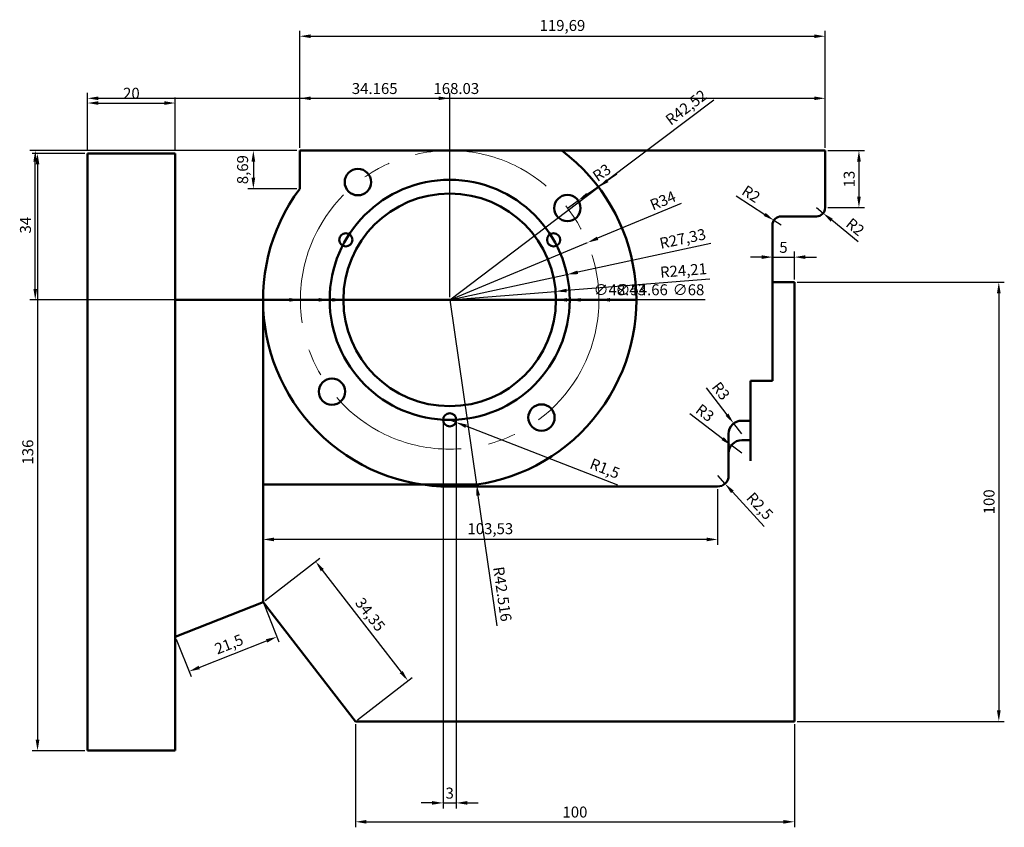
# Model space of a CAD drawing. Units: millimetres. Extents: x 1194 to 1920, y 1729 to 2086.
# Tile 4 of 5: x 1485 to 1709, y 1898 to 2082. Entities that reach past the tile are written whole.
import ezdxf

# ---------------------------------------------------------------- set-up
doc = ezdxf.new("R2010")
doc.units = ezdxf.units.MM
doc.linetypes.add('CENTER', pattern=[50.8, 31.75, -6.35, 6.35, -6.35])
for name, color, linetype, lineweight in [('M-CNTR', 1, 'CENTER', 18), ('M-DIMS', 2, 'Continuous', 25), ('M-OUTL', 7, 'Continuous', 50)]:
    doc.layers.add(name, color=color, linetype=linetype, lineweight=lineweight)
doc.styles.get("Standard").update_dxf_attribs({"font": 'arial.ttf'})
doc.dimstyles.new('ISO-25', dxfattribs={"dimtxt": 2.5, "dimasz": 2.5, "dimexe": 1.25, "dimexo": 0.625, "dimtad": 1, "dimtxsty": 'Standard', "dimcen": 2.5, "dimadec": 0, "dimazin": 0, "dimtfac": 1, "dimtmove": 0, "dimatfit": 3, "dimfxl": 1, "dimarcsym": 0})

# ---------------------------------------------------------------- blocks, each defined once
blk = doc.blocks.new('*U5')
blk.add_circle((0, 0), 1.5)
blk = doc.blocks.new('*U6')
at = {"layer": 'M-OUTL', "color": 0, "linetype": 'ByBlock', "lineweight": -2, "transparency": 16777216}
for p, rotation in [((1558.99, 2031.94), 240), ((1606.33, 2031.94), 119.9999999999999)]:
    blk.add_blockref('*U5', p, dxfattribs=dict(at, rotation=rotation))
blk.add_blockref('*U5', (1582.66, 1990.95), dxfattribs=at)
blk = doc.blocks.new('*U7')
blk.add_circle((0, 0), 3)
blk = doc.blocks.new('*U8')
at = {"layer": 'M-OUTL', "color": 0, "linetype": 'ByBlock', "lineweight": -2, "transparency": 16777216}
for p, rotation in [((1561.75, 2045.09), 90), ((1555.85, 1997.37), 180), ((1603.57, 1991.47), 270)]:
    blk.add_blockref('*U7', p, dxfattribs=dict(at, rotation=rotation))
blk.add_blockref('*U7', (1609.47, 2039.19), dxfattribs=at)
blk = doc.blocks.new('*D40')
at = {"layer": 'Defpoints', "color": 0, "transparency": 16777216}
for p in [(1500.16, 2051.61), (1488.78, 1915.61), (1500.16, 1915.61)]:
    blk.add_point(p, dxfattribs=at)
at = {"layer": 'M-DIMS', "color": 0, "lineweight": -2, "transparency": 16777216}
for p, q in [((1499.54, 2051.61), (1487.53, 2051.61)), ((1488.78, 2049.11), (1488.78, 1918.11)), ((1499.54, 1915.61), (1487.53, 1915.61))]:
    blk.add_line(p, q, dxfattribs=at)
at = {"layer": 'M-DIMS', "color": 0, "transparency": 16777216}
for points in [[(1488.36, 2049.11), (1489.2, 2049.11), (1488.78, 2051.61)], [(1488.36, 1918.11), (1489.2, 1918.11), (1488.78, 1915.61)]]:
    blk.add_solid(points, dxfattribs=at)
at = {"layer": 'M-DIMS', "color": 0, "transparency": 16777216, "insert": (1486.88, 1983.61), "char_height": 2.5, "attachment_point": 5, "rotation": 90}
blk.add_mtext('136', dxfattribs=at)
blk = doc.blocks.new('*D41')
at = {"layer": 'Defpoints', "color": 0, "transparency": 16777216}
for p in [(1520.16, 2063.1), (1500.16, 2051.61), (1520.16, 2051.61)]:
    blk.add_point(p, dxfattribs=at)
at = {"layer": 'M-DIMS', "color": 0, "lineweight": -2, "transparency": 16777216}
for p, q in [((1500.16, 2052.24), (1500.16, 2064.35)), ((1520.16, 2052.24), (1520.16, 2064.35)), ((1502.66, 2063.1), (1517.66, 2063.1))]:
    blk.add_line(p, q, dxfattribs=at)
at = {"layer": 'M-DIMS', "color": 0, "transparency": 16777216}
for points in [[(1502.66, 2063.51), (1502.66, 2062.68), (1500.16, 2063.1)], [(1517.66, 2063.51), (1517.66, 2062.68), (1520.16, 2063.1)]]:
    blk.add_solid(points, dxfattribs=at)
at = {"layer": 'M-DIMS', "color": 0, "transparency": 16777216, "insert": (1510.16, 2065), "char_height": 2.5, "attachment_point": 5}
blk.add_mtext('20', dxfattribs=at)
blk = doc.blocks.new('*D42')
at = {"layer": 'Defpoints', "color": 0, "transparency": 16777216}
for p in [(1540.16, 1949.44), (1520.16, 1941.56), (1543.28, 1941.52)]:
    blk.add_point(p, dxfattribs=at)
at = {"layer": 'M-DIMS', "color": 0, "lineweight": -2, "transparency": 16777216}
for p, q in [((1540.39, 1948.86), (1543.74, 1940.36)), ((1520.39, 1940.97), (1523.74, 1932.48)), ((1525.61, 1934.56), (1540.96, 1940.61))]:
    blk.add_line(p, q, dxfattribs=at)
at = {"layer": 'M-DIMS', "color": 0, "transparency": 16777216}
for points in [[(1540.8, 1941), (1541.11, 1940.22), (1543.28, 1941.52)], [(1525.46, 1934.94), (1525.76, 1934.17), (1523.28, 1933.64)]]:
    blk.add_solid(points, dxfattribs=at)
at = {"layer": 'M-DIMS', "color": 0, "transparency": 16777216, "insert": (1532.5, 1939.56), "char_height": 2.5, "attachment_point": 5, "rotation": 21.5204}
blk.add_mtext('21,5', dxfattribs=at)
blk = doc.blocks.new('*D43')
at = {"layer": 'Defpoints', "color": 0, "transparency": 16777216}
for p in [(1540.16, 1949.44), (1573.15, 1931.54), (1561.19, 1922.28)]:
    blk.add_point(p, dxfattribs=at)
at = {"layer": 'M-DIMS', "color": 0, "lineweight": -2, "transparency": 16777216}
for p, q in [((1540.66, 1949.82), (1553.11, 1959.46)), ((1553.65, 1956.72), (1571.62, 1933.51)), ((1561.68, 1922.66), (1574.14, 1932.3))]:
    blk.add_line(p, q, dxfattribs=at)
at = {"layer": 'M-DIMS', "color": 0, "transparency": 16777216}
for points in [[(1553.98, 1956.98), (1553.32, 1956.47), (1552.12, 1958.7)], [(1571.95, 1933.77), (1571.29, 1933.26), (1573.15, 1931.54)]]:
    blk.add_solid(points, dxfattribs=at)
at = {"layer": 'M-DIMS', "color": 0, "transparency": 16777216, "insert": (1564.32, 1946.42), "char_height": 2.5, "attachment_point": 5, "rotation": 307.7411}
blk.add_mtext('34,35', dxfattribs=at)
blk = doc.blocks.new('*D44')
at = {"layer": 'Defpoints', "color": 0, "transparency": 16777216}
for p in [(1561.19, 1922.28), (1661.19, 1922.28), (1661.19, 1899.41)]:
    blk.add_point(p, dxfattribs=at)
at = {"layer": 'M-DIMS', "color": 0, "lineweight": -2, "transparency": 16777216}
for p, q in [((1561.19, 1921.65), (1561.19, 1898.16)), ((1661.19, 1921.65), (1661.19, 1898.16)), ((1563.69, 1899.41), (1658.69, 1899.41))]:
    blk.add_line(p, q, dxfattribs=at)
at = {"layer": 'M-DIMS', "color": 0, "transparency": 16777216}
for points in [[(1563.69, 1899.82), (1563.69, 1898.99), (1561.19, 1899.41)], [(1658.69, 1899.82), (1658.69, 1898.99), (1661.19, 1899.41)]]:
    blk.add_solid(points, dxfattribs=at)
at = {"layer": 'M-DIMS', "color": 0, "transparency": 16777216, "insert": (1611.19, 1901.31), "char_height": 2.5, "attachment_point": 5}
blk.add_mtext('100', dxfattribs=at)
blk = doc.blocks.new('*D45')
at = {"layer": 'Defpoints', "color": 0, "transparency": 16777216}
for p in [(1668.19, 2078.31), (1548.5, 2052.28), (1668.19, 2052.28)]:
    blk.add_point(p, dxfattribs=at)
at = {"layer": 'M-DIMS', "color": 0, "lineweight": -2, "transparency": 16777216}
for p, q in [((1548.5, 2052.9), (1548.5, 2079.56)), ((1668.19, 2052.9), (1668.19, 2079.56)), ((1551, 2078.31), (1665.69, 2078.31))]:
    blk.add_line(p, q, dxfattribs=at)
at = {"layer": 'M-DIMS', "color": 0, "transparency": 16777216}
for points in [[(1551, 2078.73), (1551, 2077.89), (1548.5, 2078.31)], [(1665.69, 2078.73), (1665.69, 2077.89), (1668.19, 2078.31)]]:
    blk.add_solid(points, dxfattribs=at)
at = {"layer": 'M-DIMS', "color": 0, "transparency": 16777216, "insert": (1608.34, 2080.44), "char_height": 2.5, "attachment_point": 5}
blk.add_mtext('119,69', dxfattribs=at)
blk = doc.blocks.new('*D46')
at = {"layer": 'Defpoints', "color": 0, "transparency": 16777216}
for p in [(1668.19, 2052.28), (1668.19, 2039.28), (1675.88, 2039.28)]:
    blk.add_point(p, dxfattribs=at)
at = {"layer": 'M-DIMS', "color": 0, "lineweight": -2, "transparency": 16777216}
for p, q in [((1668.81, 2052.28), (1677.13, 2052.28)), ((1675.88, 2049.78), (1675.88, 2041.78)), ((1668.81, 2039.28), (1677.13, 2039.28))]:
    blk.add_line(p, q, dxfattribs=at)
at = {"layer": 'M-DIMS', "color": 0, "transparency": 16777216}
for points in [[(1675.46, 2049.78), (1676.3, 2049.78), (1675.88, 2052.28)], [(1675.46, 2041.78), (1676.3, 2041.78), (1675.88, 2039.28)]]:
    blk.add_solid(points, dxfattribs=at)
at = {"layer": 'M-DIMS', "color": 0, "transparency": 16777216, "insert": (1673.98, 2045.78), "char_height": 2.5, "attachment_point": 5, "rotation": 90}
blk.add_mtext('13', dxfattribs=at)
blk = doc.blocks.new('*D47')
at = {"layer": 'Defpoints', "color": 0, "transparency": 16777216}
for p in [(1666.19, 2039.28), (1667.73, 2038.01)]:
    blk.add_point(p, dxfattribs=at)
at = {"layer": 'M-DIMS', "color": 0, "lineweight": -2, "transparency": 16777216}
for p, q in [((1666.19, 2039.28), (1667.73, 2038.01)), ((1675.67, 2031.51), (1669.67, 2036.43))]:
    blk.add_line(p, q, dxfattribs=at)
at = {"layer": 'M-DIMS', "color": 0, "transparency": 16777216}
blk.add_solid([(1669.93, 2036.75), (1669.4, 2036.1), (1667.73, 2038.01)], dxfattribs=at)
at = {"layer": 'M-DIMS', "color": 0, "transparency": 16777216, "insert": (1674.83, 2034.63), "char_height": 2.5, "attachment_point": 5, "rotation": 320.6916}
blk.add_mtext('R2', dxfattribs=at)
blk = doc.blocks.new('*D48')
at = {"layer": 'Defpoints', "color": 0, "transparency": 16777216}
for p in [(1656.51, 2036.37), (1658.19, 2035.28)]:
    blk.add_point(p, dxfattribs=at)
at = {"layer": 'M-DIMS', "color": 0, "lineweight": -2, "transparency": 16777216}
for p, q in [((1647.92, 2041.98), (1654.42, 2037.74)), ((1658.19, 2035.28), (1656.51, 2036.37))]:
    blk.add_line(p, q, dxfattribs=at)
at = {"layer": 'M-DIMS', "color": 0, "transparency": 16777216}
blk.add_solid([(1654.65, 2038.09), (1654.19, 2037.39), (1656.51, 2036.37)], dxfattribs=at)
at = {"layer": 'M-DIMS', "color": 0, "transparency": 16777216, "insert": (1651.15, 2042.12), "char_height": 2.5, "attachment_point": 5, "rotation": 326.8616}
blk.add_mtext('R2', dxfattribs=at)
blk = doc.blocks.new('*D49')
at = {"layer": 'Defpoints', "color": 0, "transparency": 16777216}
for p in [(1661.19, 2022.28), (1661.19, 1922.28), (1707.74, 1922.28)]:
    blk.add_point(p, dxfattribs=at)
at = {"layer": 'M-DIMS', "color": 0, "lineweight": -2, "transparency": 16777216}
for p, q in [((1661.81, 2022.28), (1708.99, 2022.28)), ((1707.74, 2019.78), (1707.74, 1924.78)), ((1661.81, 1922.28), (1708.99, 1922.28))]:
    blk.add_line(p, q, dxfattribs=at)
at = {"layer": 'M-DIMS', "color": 0, "transparency": 16777216}
for points in [[(1707.32, 2019.78), (1708.16, 2019.78), (1707.74, 2022.28)], [(1707.32, 1924.78), (1708.16, 1924.78), (1707.74, 1922.28)]]:
    blk.add_solid(points, dxfattribs=at)
at = {"layer": 'M-DIMS', "color": 0, "transparency": 16777216, "insert": (1705.84, 1972.28), "char_height": 2.5, "attachment_point": 5, "rotation": 90}
blk.add_mtext('100', dxfattribs=at)
blk = doc.blocks.new('*D50')
at = {"layer": 'Defpoints', "color": 0, "transparency": 16777216}
for p in [(1661.19, 2028.01), (1656.19, 2022.28), (1661.19, 2022.28)]:
    blk.add_point(p, dxfattribs=at)
at = {"layer": 'M-DIMS', "color": 0, "lineweight": -2, "transparency": 16777216}
for p, q in [((1653.69, 2028.01), (1651.19, 2028.01)), ((1656.19, 2022.9), (1656.19, 2029.26)), ((1656.19, 2028.01), (1661.19, 2028.01)), ((1661.19, 2022.9), (1661.19, 2029.26)), ((1663.69, 2028.01), (1666.19, 2028.01))]:
    blk.add_line(p, q, dxfattribs=at)
at = {"layer": 'M-DIMS', "color": 0, "transparency": 16777216}
for points in [[(1653.69, 2028.43), (1653.69, 2027.59), (1656.19, 2028.01)], [(1663.69, 2028.43), (1663.69, 2027.59), (1661.19, 2028.01)]]:
    blk.add_solid(points, dxfattribs=at)
at = {"layer": 'M-DIMS', "color": 0, "transparency": 16777216, "insert": (1658.69, 2029.91), "char_height": 2.5, "attachment_point": 5}
blk.add_mtext('5', dxfattribs=at)
blk = doc.blocks.new('*D51')
at = {"layer": 'Defpoints', "color": 0, "transparency": 16777216}
for p in [(1540.16, 1976.21), (1643.69, 1975.76), (1540.16, 1963.71)]:
    blk.add_point(p, dxfattribs=at)
at = {"layer": 'M-DIMS', "color": 0, "lineweight": -2, "transparency": 16777216}
for p, q in [((1540.16, 1975.58), (1540.16, 1962.46)), ((1643.69, 1975.14), (1643.69, 1962.46)), ((1641.19, 1963.71), (1542.66, 1963.71))]:
    blk.add_line(p, q, dxfattribs=at)
at = {"layer": 'M-DIMS', "color": 0, "transparency": 16777216}
for points in [[(1542.66, 1964.13), (1542.66, 1963.29), (1540.16, 1963.71)], [(1641.19, 1964.13), (1641.19, 1963.29), (1643.69, 1963.71)]]:
    blk.add_solid(points, dxfattribs=at)
at = {"layer": 'M-DIMS', "color": 0, "transparency": 16777216, "insert": (1591.92, 1965.84), "char_height": 2.5, "attachment_point": 5}
blk.add_mtext('103,53', dxfattribs=at)
blk = doc.blocks.new('*D52')
at = {"layer": 'Defpoints', "color": 0, "transparency": 16777216}
for p in [(1647.35, 1990.14), (1649.19, 1987.76)]:
    blk.add_point(p, dxfattribs=at)
at = {"layer": 'M-DIMS', "color": 0, "lineweight": -2, "transparency": 16777216}
for p, q in [((1641.06, 1998.27), (1645.82, 1992.11)), ((1649.19, 1987.76), (1647.35, 1990.14))]:
    blk.add_line(p, q, dxfattribs=at)
at = {"layer": 'M-DIMS', "color": 0, "transparency": 16777216}
blk.add_solid([(1646.15, 1992.37), (1645.49, 1991.86), (1647.35, 1990.14)], dxfattribs=at)
at = {"layer": 'M-DIMS', "color": 0, "transparency": 16777216, "insert": (1644.18, 1997.34), "char_height": 2.5, "attachment_point": 5, "rotation": 307.7239}
blk.add_mtext('R3', dxfattribs=at)
blk = doc.blocks.new('*D53')
at = {"layer": 'Defpoints', "color": 0, "transparency": 16777216}
for p in [(1646.81, 1985.15), (1649.19, 1983.33)]:
    blk.add_point(p, dxfattribs=at)
at = {"layer": 'M-DIMS', "color": 0, "lineweight": -2, "transparency": 16777216}
for p, q in [((1637.36, 1992.39), (1644.82, 1986.67)), ((1649.19, 1983.33), (1646.81, 1985.15))]:
    blk.add_line(p, q, dxfattribs=at)
at = {"layer": 'M-DIMS', "color": 0, "transparency": 16777216}
blk.add_solid([(1645.07, 1987), (1644.57, 1986.34), (1646.81, 1985.15)], dxfattribs=at)
at = {"layer": 'M-DIMS', "color": 0, "transparency": 16777216, "insert": (1640.61, 1992.29), "char_height": 2.5, "attachment_point": 5, "rotation": 322.5412}
blk.add_mtext('R3', dxfattribs=at)
blk = doc.blocks.new('*D54')
at = {"layer": 'Defpoints', "color": 0, "transparency": 16777216}
for p in [(1643.69, 1978.26), (1645.37, 1976.41)]:
    blk.add_point(p, dxfattribs=at)
at = {"layer": 'M-DIMS', "color": 0, "lineweight": -2, "transparency": 16777216}
for p, q in [((1643.69, 1978.26), (1645.37, 1976.41)), ((1654.26, 1966.64), (1647.05, 1974.56))]:
    blk.add_line(p, q, dxfattribs=at)
at = {"layer": 'M-DIMS', "color": 0, "transparency": 16777216}
blk.add_solid([(1647.36, 1974.84), (1646.74, 1974.28), (1645.37, 1976.41)], dxfattribs=at)
at = {"layer": 'M-DIMS', "color": 0, "transparency": 16777216, "insert": (1653.07, 1971.11), "char_height": 2.5, "attachment_point": 5, "rotation": 312.2746}
blk.add_mtext('R2,5', dxfattribs=at)
blk = doc.blocks.new('*D55')
at = {"layer": 'Defpoints', "color": 0, "transparency": 16777216}
for p in [(1616.57, 2043.93), (1582.66, 2018.28)]:
    blk.add_point(p, dxfattribs=at)
at = {"layer": 'M-DIMS', "color": 0, "lineweight": -2, "transparency": 16777216}
for p, q in [((1642.81, 2063.78), (1618.56, 2045.44)), ((1582.66, 2018.28), (1616.57, 2043.93))]:
    blk.add_line(p, q, dxfattribs=at)
at = {"layer": 'M-DIMS', "color": 0, "transparency": 16777216}
blk.add_solid([(1618.31, 2045.77), (1618.81, 2045.1), (1616.57, 2043.93)], dxfattribs=at)
at = {"layer": 'M-DIMS', "color": 0, "transparency": 16777216, "insert": (1636.72, 2061.84), "char_height": 2.5, "attachment_point": 5, "rotation": 37.1061}
blk.add_mtext('R42,52', dxfattribs=at)
blk = doc.blocks.new('*D56')
at = {"layer": 'Defpoints', "color": 0, "transparency": 16777216}
for p in [(1614.06, 2031.33), (1582.66, 2018.28)]:
    blk.add_point(p, dxfattribs=at)
at = {"layer": 'M-DIMS', "color": 0, "lineweight": -2, "transparency": 16777216}
for p, q in [((1635.4, 2040.21), (1616.36, 2032.29)), ((1582.66, 2018.28), (1614.06, 2031.33))]:
    blk.add_line(p, q, dxfattribs=at)
at = {"layer": 'M-DIMS', "color": 0, "transparency": 16777216}
blk.add_solid([(1616.2, 2032.68), (1616.52, 2031.91), (1614.06, 2031.33)], dxfattribs=at)
at = {"layer": 'M-DIMS', "color": 0, "transparency": 16777216, "insert": (1631.34, 2040.58), "char_height": 2.5, "attachment_point": 5, "rotation": 22.5772}
blk.add_mtext('R34', dxfattribs=at)
blk = doc.blocks.new('*D57')
at = {"layer": 'Defpoints', "color": 0, "transparency": 16777216}
for p in [(1609.38, 2024.03), (1582.66, 2018.28)]:
    blk.add_point(p, dxfattribs=at)
at = {"layer": 'M-DIMS', "color": 0, "lineweight": -2, "transparency": 16777216}
for p, q in [((1642.15, 2031.08), (1611.82, 2024.55)), ((1582.66, 2018.28), (1609.38, 2024.03))]:
    blk.add_line(p, q, dxfattribs=at)
at = {"layer": 'M-DIMS', "color": 0, "transparency": 16777216}
blk.add_solid([(1611.74, 2024.96), (1611.91, 2024.14), (1609.38, 2024.03)], dxfattribs=at)
at = {"layer": 'M-DIMS', "color": 0, "transparency": 16777216, "insert": (1635.8, 2031.89), "char_height": 2.5, "attachment_point": 5, "rotation": 12.1415}
blk.add_mtext('R27,33', dxfattribs=at)
blk = doc.blocks.new('*D58')
at = {"layer": 'Defpoints', "color": 0, "transparency": 16777216}
for p in [(1606.8, 2020.2), (1582.66, 2018.28)]:
    blk.add_point(p, dxfattribs=at)
at = {"layer": 'M-DIMS', "color": 0, "lineweight": -2, "transparency": 16777216}
for p, q in [((1641.89, 2023), (1609.29, 2020.4)), ((1582.66, 2018.28), (1606.8, 2020.2))]:
    blk.add_line(p, q, dxfattribs=at)
at = {"layer": 'M-DIMS', "color": 0, "transparency": 16777216}
blk.add_solid([(1609.26, 2020.82), (1609.32, 2019.99), (1606.8, 2020.2)], dxfattribs=at)
at = {"layer": 'M-DIMS', "color": 0, "transparency": 16777216, "insert": (1635.94, 2024.66), "char_height": 2.5, "attachment_point": 5, "rotation": 4.5586}
blk.add_mtext('R24,21', dxfattribs=at)
blk = doc.blocks.new('*D59')
at = {"layer": 'Defpoints', "color": 0, "transparency": 16777216}
for p in [(1611.94, 2040.89), (1609.47, 2039.19)]:
    blk.add_point(p, dxfattribs=at)
at = {"layer": 'M-DIMS', "color": 0, "lineweight": -2, "transparency": 16777216}
for p, q in [((1620.74, 2046.93), (1614, 2042.3)), ((1609.47, 2039.19), (1611.94, 2040.89))]:
    blk.add_line(p, q, dxfattribs=at)
at = {"layer": 'M-DIMS', "color": 0, "transparency": 16777216}
blk.add_solid([(1613.77, 2042.65), (1614.24, 2041.96), (1611.94, 2040.89)], dxfattribs=at)
at = {"layer": 'M-DIMS', "color": 0, "transparency": 16777216, "insert": (1617.48, 2047), "char_height": 2.5, "attachment_point": 5, "rotation": 34.5057}
blk.add_mtext('R3', dxfattribs=at)
blk = doc.blocks.new('*D60')
at = {"layer": 'Defpoints', "color": 0, "transparency": 16777216}
for p in [(1582.66, 1990.95), (1584.06, 1990.4)]:
    blk.add_point(p, dxfattribs=at)
at = {"layer": 'M-DIMS', "color": 0, "lineweight": -2, "transparency": 16777216}
for p, q in [((1582.66, 1990.95), (1584.06, 1990.4)), ((1620.95, 1976.11), (1586.39, 1989.5))]:
    blk.add_line(p, q, dxfattribs=at)
at = {"layer": 'M-DIMS', "color": 0, "transparency": 16777216}
blk.add_solid([(1586.54, 1989.89), (1586.24, 1989.11), (1584.06, 1990.4)], dxfattribs=at)
at = {"layer": 'M-DIMS', "color": 0, "transparency": 16777216, "insert": (1617.89, 1979.58), "char_height": 2.5, "attachment_point": 5, "rotation": 338.8182}
blk.add_mtext('R1,5', dxfattribs=at)
blk = doc.blocks.new('*D61')
at = {"layer": 'Defpoints', "color": 0, "transparency": 16777216}
for p in [(1548.5, 2052.28), (1537.94, 2043.58), (1548.5, 2043.58)]:
    blk.add_point(p, dxfattribs=at)
at = {"layer": 'M-DIMS', "color": 0, "lineweight": -2, "transparency": 16777216}
for p, q in [((1547.87, 2052.28), (1536.69, 2052.28)), ((1537.94, 2049.78), (1537.94, 2046.08)), ((1547.87, 2043.58), (1536.69, 2043.58))]:
    blk.add_line(p, q, dxfattribs=at)
at = {"layer": 'M-DIMS', "color": 0, "transparency": 16777216}
for points in [[(1537.53, 2049.78), (1538.36, 2049.78), (1537.94, 2052.28)], [(1537.53, 2046.08), (1538.36, 2046.08), (1537.94, 2043.58)]]:
    blk.add_solid(points, dxfattribs=at)
at = {"layer": 'M-DIMS', "color": 0, "transparency": 16777216, "insert": (1535.82, 2047.93), "char_height": 2.5, "attachment_point": 5, "rotation": 90}
blk.add_mtext('8,69', dxfattribs=at)
blk = doc.blocks.new('*D137')
at = {"layer": 'Defpoints', "color": 0, "transparency": 16777216}
for p in [(1581.16, 1990.95), (1584.16, 1990.95), (1584.16, 1903.71)]:
    blk.add_point(p, dxfattribs=at)
at = {"layer": 'M-DIMS', "color": 0, "lineweight": -2, "transparency": 16777216}
for p, q in [((1581.16, 1990.32), (1581.16, 1902.46)), ((1584.16, 1990.32), (1584.16, 1902.46)), ((1578.66, 1903.71), (1576.16, 1903.71)), ((1581.16, 1903.71), (1584.16, 1903.71)), ((1586.66, 1903.71), (1589.16, 1903.71))]:
    blk.add_line(p, q, dxfattribs=at)
at = {"layer": 'M-DIMS', "color": 0, "transparency": 16777216}
for points in [[(1578.66, 1904.13), (1578.66, 1903.3), (1581.16, 1903.71)], [(1586.66, 1904.13), (1586.66, 1903.3), (1584.16, 1903.71)]]:
    blk.add_solid(points, dxfattribs=at)
at = {"layer": 'M-DIMS', "color": 0, "transparency": 16777216, "insert": (1582.66, 1905.62), "char_height": 2.5, "attachment_point": 5}
blk.add_mtext('3', dxfattribs=at)
blk = doc.blocks.new('*D139')
at = {"layer": 'Defpoints', "color": 0, "transparency": 16777216}
for p in [(1668.19, 2064.18), (1668.19, 2052.28), (1500.16, 2051.61)]:
    blk.add_point(p, dxfattribs=at)
at = {"layer": 'M-DIMS', "color": 0, "lineweight": -2, "transparency": 16777216}
for p, q in [((1500.16, 2052.24), (1500.16, 2065.43)), ((1502.66, 2064.18), (1665.69, 2064.18)), ((1668.19, 2052.9), (1668.19, 2065.43))]:
    blk.add_line(p, q, dxfattribs=at)
at = {"layer": 'M-DIMS', "color": 0, "transparency": 16777216}
for points in [[(1502.66, 2064.59), (1502.66, 2063.76), (1500.16, 2064.18)], [(1665.69, 2064.59), (1665.69, 2063.76), (1668.19, 2064.18)]]:
    blk.add_solid(points, dxfattribs=at)
at = {"layer": 'M-DIMS', "color": 0, "transparency": 16777216, "insert": (1584.17, 2066.08), "char_height": 2.5, "attachment_point": 5}
blk.add_mtext('168.03', dxfattribs=at)
blk = doc.blocks.new('*D140')
at = {"layer": 'Defpoints', "color": 0, "transparency": 16777216}
for p in [(1582.66, 2064.18), (1548.5, 2052.28), (1582.66, 2018.28)]:
    blk.add_point(p, dxfattribs=at)
at = {"layer": 'M-DIMS', "color": 0, "lineweight": -2, "transparency": 16777216}
for p, q in [((1548.5, 2052.9), (1548.5, 2065.43)), ((1551, 2064.18), (1580.16, 2064.18)), ((1582.66, 2018.9), (1582.66, 2065.43))]:
    blk.add_line(p, q, dxfattribs=at)
at = {"layer": 'M-DIMS', "color": 0, "transparency": 16777216}
for points in [[(1551, 2064.59), (1551, 2063.76), (1548.5, 2064.18)], [(1580.16, 2064.59), (1580.16, 2063.76), (1582.66, 2064.18)]]:
    blk.add_solid(points, dxfattribs=at)
at = {"layer": 'M-DIMS', "color": 0, "transparency": 16777216, "insert": (1565.58, 2066.08), "char_height": 2.5, "attachment_point": 5}
blk.add_mtext('34.165', dxfattribs=at)
blk = doc.blocks.new('*D141')
at = {"layer": 'Defpoints', "color": 0, "transparency": 16777216}
for p in [(1488.26, 2052.28), (1548.5, 2052.28), (1582.66, 2018.28)]:
    blk.add_point(p, dxfattribs=at)
at = {"layer": 'M-DIMS', "color": 0, "lineweight": -2, "transparency": 16777216}
for p, q in [((1547.87, 2052.28), (1487.01, 2052.28)), ((1488.26, 2020.78), (1488.26, 2049.78)), ((1582.04, 2018.28), (1487.01, 2018.28))]:
    blk.add_line(p, q, dxfattribs=at)
at = {"layer": 'M-DIMS', "color": 0, "transparency": 16777216}
for points in [[(1487.84, 2049.78), (1488.68, 2049.78), (1488.26, 2052.28)], [(1487.84, 2020.78), (1488.68, 2020.78), (1488.26, 2018.28)]]:
    blk.add_solid(points, dxfattribs=at)
at = {"layer": 'M-DIMS', "color": 0, "transparency": 16777216, "insert": (1486.36, 2035.28), "char_height": 2.5, "attachment_point": 5, "rotation": 90}
blk.add_mtext('34', dxfattribs=at)
blk = doc.blocks.new('*D145')
at = {"layer": 'Defpoints', "color": 0, "transparency": 16777216}
for p in [(1582.66, 2018.28), (1588.79, 1976.21)]:
    blk.add_point(p, dxfattribs=at)
at = {"layer": 'M-DIMS', "color": 0, "lineweight": -2, "transparency": 16777216}
for p, q in [((1582.66, 2018.28), (1588.79, 1976.21)), ((1593.48, 1944.03), (1589.15, 1973.73))]:
    blk.add_line(p, q, dxfattribs=at)
at = {"layer": 'M-DIMS', "color": 0, "transparency": 16777216}
blk.add_solid([(1589.56, 1973.79), (1588.74, 1973.67), (1588.79, 1976.21)], dxfattribs=at)
at = {"layer": 'M-DIMS', "color": 0, "transparency": 16777216, "insert": (1594.35, 1951.24), "char_height": 2.5, "attachment_point": 5, "rotation": 278.2873}
blk.add_mtext('R42.516', dxfattribs=at)
blk = doc.blocks.new('*D146')
at = {"layer": 'Defpoints', "color": 0, "transparency": 16777216}
for p in [(1548.66, 2018.28), (1616.66, 2018.28)]:
    blk.add_point(p, dxfattribs=at)
at = {"layer": 'M-DIMS', "color": 0, "lineweight": -2, "transparency": 16777216}
for p, q in [((1546.16, 2018.28), (1543.66, 2018.28)), ((1548.66, 2018.28), (1616.66, 2018.28)), ((1640.84, 2018.28), (1619.16, 2018.28))]:
    blk.add_line(p, q, dxfattribs=at)
at = {"layer": 'M-DIMS', "color": 0, "transparency": 16777216}
for points in [[(1546.16, 2018.69), (1546.16, 2017.86), (1548.66, 2018.28)], [(1619.16, 2018.69), (1619.16, 2017.86), (1616.66, 2018.28)]]:
    blk.add_solid(points, dxfattribs=at)
at = {"layer": 'M-DIMS', "color": 0, "transparency": 16777216, "insert": (1637.06, 2020.25), "char_height": 2.5, "attachment_point": 5, "rotation": 0.0001}
blk.add_mtext('∅68', dxfattribs=at)
blk = doc.blocks.new('*D147')
at = {"layer": 'Defpoints', "color": 0, "transparency": 16777216}
for p in [(1555.33, 2018.28), (1609.99, 2018.28)]:
    blk.add_point(p, dxfattribs=at)
at = {"layer": 'M-DIMS', "color": 0, "lineweight": -2, "transparency": 16777216}
for p, q in [((1552.83, 2018.28), (1550.33, 2018.28)), ((1555.33, 2018.28), (1609.99, 2018.28)), ((1632.59, 2018.28), (1612.49, 2018.28))]:
    blk.add_line(p, q, dxfattribs=at)
at = {"layer": 'M-DIMS', "color": 0, "transparency": 16777216}
for points in [[(1552.83, 2018.69), (1552.83, 2017.86), (1555.33, 2018.28)], [(1612.49, 2018.69), (1612.49, 2017.86), (1609.99, 2018.28)]]:
    blk.add_solid(points, dxfattribs=at)
at = {"layer": 'M-DIMS', "color": 0, "transparency": 16777216, "insert": (1626.39, 2020.25), "char_height": 2.5, "attachment_point": 5, "rotation": 0.0002}
blk.add_mtext('∅54.66', dxfattribs=at)
blk = doc.blocks.new('*D148')
at = {"layer": 'Defpoints', "color": 0, "transparency": 16777216}
for p in [(1558.45, 2018.28), (1606.88, 2018.28)]:
    blk.add_point(p, dxfattribs=at)
at = {"layer": 'M-DIMS', "color": 0, "lineweight": -2, "transparency": 16777216}
for p, q in [((1555.95, 2018.28), (1553.45, 2018.28)), ((1558.45, 2018.28), (1606.88, 2018.28)), ((1627.61, 2018.28), (1609.38, 2018.28))]:
    blk.add_line(p, q, dxfattribs=at)
at = {"layer": 'M-DIMS', "color": 0, "transparency": 16777216}
for points in [[(1555.95, 2018.69), (1555.95, 2017.86), (1558.45, 2018.28)], [(1609.38, 2018.69), (1609.38, 2017.86), (1606.88, 2018.28)]]:
    blk.add_solid(points, dxfattribs=at)
at = {"layer": 'M-DIMS', "color": 0, "transparency": 16777216, "insert": (1621.4, 2020.25), "char_height": 2.5, "attachment_point": 5, "rotation": 0.0002}
blk.add_mtext('∅48.43', dxfattribs=at)

msp = doc.modelspace()

# ---------------------------------------------------------------- linework, layer by layer
at = {"layer": 'M-CNTR'}
msp.add_circle((1582.6609, 2018.2779), 34, dxfattribs=at)
at = {"layer": 'M-OUTL'}
for p, q in [((1548.4964, 2043.5834), (1548.4964, 2052.2779)), ((1582.6609, 2052.2779), (1548.4964, 2052.2779)), ((1582.6609, 2052.2779), (1608.187, 2052.2779)), ((1608.187, 2052.2779), (1668.187, 2052.2779)), ((1668.187, 2052.2779), (1668.187, 2039.2779)), ((1500.1609, 2051.6148), (1500.1609, 1915.6148)), ((1520.1609, 2051.6148), (1500.1609, 2051.6148)), ((1520.1609, 1915.6148), (1520.1609, 2051.6148)), ((1656.187, 2037.2779), (1656.187, 2037.2779)), ((1666.187, 2037.2779), (1658.187, 2037.2779)), ((1656.187, 2035.2779), (1656.187, 1999.8538)), ((1656.187, 2035.2779), (1656.187, 2022.2779)), ((1656.187, 2022.2779), (1661.187, 2022.2779)), ((1661.187, 2022.2779), (1661.187, 1922.2779)), ((1520.1609, 2018.2779), (1625.1765, 2018.2779)), ((1520.1609, 2018.2779), (1540.1609, 2018.2779)), ((1540.1609, 2018.2779), (1540.1609, 1949.4422)), ((1656.187, 1999.8538), (1651.187, 1999.8538)), ((1651.187, 1999.8538), (1651.187, 1981.5982)), ((1649.187, 1990.7623), (1651.187, 1990.7623)), ((1646.187, 1983.3258), (1646.187, 1987.7623)), ((1649.187, 1986.3258), (1651.187, 1986.3258)), ((1646.187, 1978.2623), (1646.187, 1983.3258)), ((1588.7891, 1976.2063), (1540.1609, 1976.2063)), ((1582.6609, 1975.7623), (1643.687, 1975.7623)), ((1540.1609, 1949.4422), (1520.1609, 1941.5557)), ((1561.187, 1922.2779), (1540.1609, 1949.4422)), ((1661.187, 1922.2779), (1561.187, 1922.2779)), ((1500.1609, 1915.6148), (1520.1609, 1915.6148))]:
    msp.add_line(p, q, dxfattribs=at)
for radius in [27.3311, 24.2146]:
    msp.add_circle((1582.6609, 2018.2779), radius, dxfattribs=at)
for centre, radius, start, end in [((1582.6609, 2018.2779), 42.5156, 143.472882, 53.101997), ((1666.187, 2039.2779), 2, 270, 0), ((1658.187, 2035.2779), 2, 90, 180), ((1649.187, 1987.7623), 3, 90, 180), ((1649.187, 1983.3258), 3, 90, 180), ((1643.687, 1978.2623), 2.5, 270, 0)]:
    msp.add_arc(centre, radius, start, end, dxfattribs=at)

# ---------------------------------------------------------------- block references
for name in ['*U8', '*U6']:
    msp.add_blockref(name, (0, 0), dxfattribs=at)

# ---------------------------------------------------------------- dimensions: what is measured, and where the dimension line sits
at = {"layer": 'M-DIMS'}
for base, p1, p2, override, picture, middle in [((1668.187, 2078.3103), (1548.4964, 2052.2779), (1668.187, 2052.2779), {"dimclrd": 0, "dimclre": 0, "dimclrt": 0}, '*D45', (1608.3417, 2080.4376)), ((1668.187, 2064.1779), (1500.1609, 2051.6148), (1668.187, 2052.2779), {"dimdec": 2, "dimlfac": 1, "dimrnd": 0, "dimzin": 0, "dimdsep": 46, "dimlunit": 2}, '*D139', (1584.1739, 2066.0802)), ((1520.1609, 2063.0975), (1500.1609, 2051.6148), (1520.1609, 2051.6148), {"dimclrd": 0, "dimclre": 0, "dimclrt": 0}, '*D41', (1510.1609, 2064.9989)), ((1582.6609, 2064.17792), (1548.49638, 2052.27792), (1582.6609, 2018.27793), {"dimdec": 3, "dimlfac": 1, "dimrnd": 0, "dimzin": 0, "dimdsep": 46, "dimlunit": 2}, '*D140', (1565.57864, 2066.08021)), ((1661.187, 2028.0112), (1656.187, 2022.2779), (1661.187, 2022.2779), {"dimclrd": 0, "dimclre": 0, "dimclrt": 0}, '*D50', (1658.687, 2029.9075)), ((1584.1609, 1903.7148), (1581.1609, 1990.9468), (1584.1609, 1990.9468), {"dimdec": 0, "dimlfac": 1, "dimrnd": 0, "dimzin": 0, "dimdsep": 46, "dimlunit": 2}, '*D137', (1582.6609, 1905.6171)), ((1540.1609, 1963.7089), (1643.687, 1975.7623), (1540.1609, 1976.2063), {"dimclrd": 0, "dimclre": 0, "dimclrt": 0}, '*D51', (1591.9239, 1965.8363)), ((1661.187, 1899.407), (1561.187, 1922.2779), (1661.187, 1922.2779), {"dimclrd": 0, "dimclre": 0, "dimclrt": 0}, '*D44', (1611.187, 1901.3085))]:
    dim = msp.add_linear_dim(base=base, p1=p1, p2=p2, dimstyle='ISO-25', override=override, dxfattribs=at)
    dim.commit()
    dim.dimension.update_dxf_attribs({"geometry": picture, "text_midpoint": middle})
for center, mpoint, override, picture, middle in [((1582.6609, 2018.2779), (1616.568, 2043.9273), {"dimclrd": 0, "dimclre": 0, "dimclrt": 0}, '*D55', (1638.0005, 2060.1402)), ((1609.4717, 2039.1868), (1611.9439, 2040.8863), {"dimclrd": 0, "dimclre": 0, "dimclrt": 0}, '*D59', (1618.5618, 2045.4355)), ((1582.6609, 2018.2779), (1614.0552, 2031.3315), {"dimclrd": 0, "dimclre": 0, "dimclrt": 0}, '*D56', (1632.072, 2038.8227)), ((1582.6609, 2018.2779), (1609.3807, 2024.0264), {"dimclrd": 0, "dimclre": 0, "dimclrt": 0}, '*D57', (1636.2474, 2029.8065)), ((1582.6609, 2018.2779), (1606.7989, 2020.2025), {"dimclrd": 0, "dimclre": 0, "dimclrt": 0}, '*D58', (1636.1127, 2022.5396)), ((1582.6609, 2018.2779), (1588.789, 1976.2062), {"dimdec": 3, "dimlfac": 1, "dimrnd": 0, "dimzin": 0, "dimdsep": 46, "dimlunit": 2}, '*D145', (1592.4658, 1950.9632)), ((1649.187, 1983.3258), (1646.8056, 1985.1504), {"dimclrd": 0, "dimclre": 0, "dimclrt": 0}, '*D53', (1639.4529, 1990.7839)), ((1582.6609, 1990.9468), (1584.0596, 1990.4048), {"dimclrd": 0, "dimclre": 0, "dimclrt": 0}, '*D60', (1617.1216, 1977.593))]:
    dim = msp.add_radius_dim(center=center, mpoint=mpoint, dimstyle='ISO-25', override=override, dxfattribs=at)
    dim.commit()
    dim.dimension.update_dxf_attribs({"geometry": picture, "text_midpoint": middle, "dimtype": 164})
for base, p1, p2, override, picture, middle in [((1488.2609, 2052.2779), (1582.6609, 2018.2779), (1548.4964, 2052.2779), {"dimdec": 0, "dimlfac": 1, "dimrnd": 0, "dimzin": 0, "dimdsep": 46, "dimlunit": 2}, '*D141', (1486.3586, 2035.2779)), ((1537.9436, 2043.5834), (1548.4964, 2052.2779), (1548.4964, 2043.5834), {"dimclrd": 0, "dimclre": 0, "dimclrt": 0}, '*D61', (1535.8162, 2047.9306)), ((1675.8815, 2039.2779), (1668.187, 2052.2779), (1668.187, 2039.2779), {"dimclrd": 0, "dimclre": 0, "dimclrt": 0}, '*D46', (1673.9793, 2045.7779)), ((1488.7801, 1915.6148), (1500.1609, 2051.6148), (1500.1609, 1915.6148), {"dimclrd": 0, "dimclre": 0, "dimclrt": 0}, '*D40', (1486.8778, 1983.6148)), ((1707.7408, 1922.2779), (1661.187, 2022.2779), (1661.187, 1922.2779), {"dimclrd": 0, "dimclre": 0, "dimclrt": 0}, '*D49', (1705.8394, 1972.2779))]:
    dim = msp.add_linear_dim(base=base, p1=p1, p2=p2, angle=90, dimstyle='ISO-25', override=override, dxfattribs=at)
    dim.commit()
    dim.dimension.update_dxf_attribs({"geometry": picture, "text_midpoint": middle})
for center, mpoint, picture, middle in [((1658.187, 2035.2779), (1656.5123, 2036.3713), '*D48', (1651.1528, 2042.1155)), ((1666.187, 2039.2779), (1667.7345, 2038.0109), '*D47', (1674.8276, 2034.6334)), ((1649.187, 1987.7623), (1647.3514, 1990.1352), '*D52', (1644.181, 1997.3427)), ((1643.687, 1978.2623), (1645.3687, 1976.4125), '*D54', (1653.0685, 1971.1054))]:
    dim = msp.add_radius_dim(center=center, mpoint=mpoint, dimstyle='ISO-25', override={"dimclrd": 0, "dimclre": 0, "dimclrt": 0}, dxfattribs=at)
    dim.commit()
    dim.dimension.update_dxf_attribs({"geometry": picture, "text_midpoint": middle})
for p1, p2, override, picture, middle in [((1548.6609, 2018.2778), (1616.6609, 2018.278), {"dimdec": 0, "dimlfac": 1, "dimrnd": 0, "dimzin": 0, "dimdsep": 46, "dimlunit": 2}, '*D146', (1637.0609, 2018.278)), ((1555.3298, 2018.2778), (1609.992, 2018.278), {"dimdec": 2, "dimlfac": 1, "dimrnd": 0, "dimzin": 0, "dimdsep": 46, "dimlunit": 2}, '*D147', (1626.3907, 2018.278)), ((1558.4463, 2018.2778), (1606.8755, 2018.278), {"dimdec": 2, "dimlfac": 1, "dimrnd": 0, "dimzin": 0, "dimdsep": 46, "dimlunit": 2}, '*D148', (1621.4042, 2018.278))]:
    dim = msp.add_diameter_dim_2p(p1=p1, p2=p2, dimstyle='ISO-25', override=override, dxfattribs=at)
    dim.commit()
    dim.dimension.update_dxf_attribs({"geometry": picture, "text_midpoint": middle, "dimtype": 163})
for p1, p2, distance, picture, middle in [((1540.1609, 1949.4422), (1561.187, 1922.2779), 15.1244, '*D43', (1564.3164, 1946.4198)), ((1520.1609, 1941.5557), (1540.1609, 1949.4422), -8.5108, '*D42', (1532.5026, 1939.5605))]:
    dim = msp.add_aligned_dim(p1=p1, p2=p2, distance=distance, dimstyle='ISO-25', override={"dimclrd": 0, "dimclre": 0, "dimclrt": 0}, dxfattribs=at)
    dim.commit()
    dim.dimension.update_dxf_attribs({"geometry": picture, "text_midpoint": middle})

doc.saveas('drawing.dxf')
